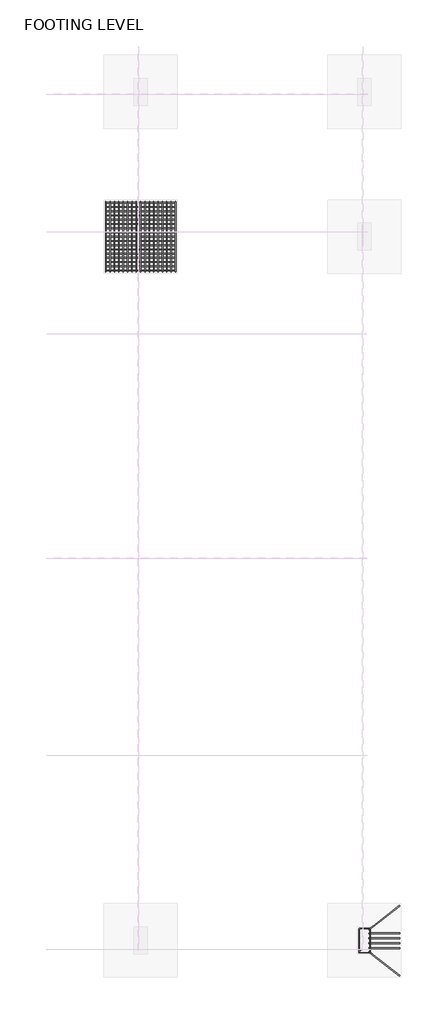
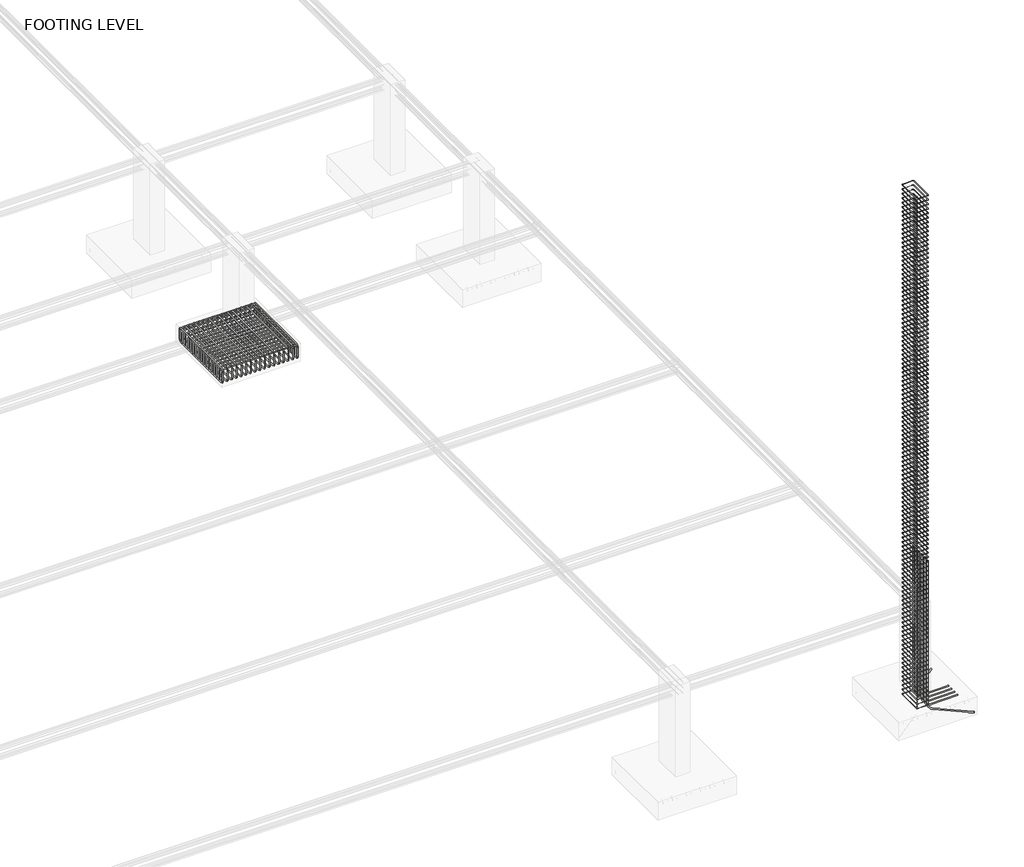
# One storey, part 9 of 19: 7 reinforcing bars.
"""IFC4 building model written with IfcOpenShell, lengths in millimetres."""

from ifc_helpers import new_model, si_unit, point, frame, origin, place, context, project, spatial, polyline, circle_curve, trimmed, segment, composite_curve, source, transform, mapped, element, save
from ifc_brep_helpers import swept_disk

model = new_model("IFC4")

# Units and contexts
model_context = context("Model", 3, world=origin())
ifc_project = project(units=[si_unit("LENGTHUNIT", "METRE", prefix="MILLI")], contexts=[model_context])

# Site, building, storey
site = spatial("IfcSite", under=ifc_project)
building = spatial("IfcBuilding", under=site)
storey = spatial("IfcBuildingStorey", under=building, Name="FOOTING LEVEL", Elevation=-3048.0)

# Reinforcing bars
placement = place(None, origin())
element("IfcReinforcingBar", 1, at=placement, inside=storey, context=model_context, shape_type="SolidModel", body=[
    swept_disk(composite_curve([segment(polyline([(32474.4469298, -27441.1521798, 1397.9656204), (32474.4469298, -27441.1521798, -3426.35)]), True, "CONTINUOUS"), segment(trimmed(circle_curve(frame((32595.5247821, -27346.5557941, -3426.35), z_axis=(0.6156614753256462, -0.7880107536067313, 0.0), x_axis=(-121.07785230000081, -94.59638569999879, 0.0)), 153.65), [point((32474.4469298, -27441.1521798, -3426.35))], [point((32595.5247821, -27346.5557941, -3580.0))], True, "CARTESIAN"), True, "CONTINUOUS"), segment(polyline([(32595.5247821, -27346.5557941, -3580.0), (33499.706152, -26640.131886, -3580.0)]), True, "CONTINUOUS")], self_intersect=False), 16.15),
])
element("IfcReinforcingBar", 2, at=placement, inside=storey, context=model_context, shape_type="SolidModel", body=[
    swept_disk(composite_curve([segment(polyline([(32473.5341356, -28221.1523853, 1369.4444311), (32473.5341356, -28221.1523853, -3426.35)]), True, "CONTINUOUS"), segment(trimmed(circle_curve(frame((32594.6119879, -28315.7487709, -3426.35), z_axis=(-0.6156614753256462, -0.7880107536067313, 0.0), x_axis=(-121.07785230000081, 94.59638560000167, 0.0)), 153.65), [point((32473.5341356, -28221.1523853, -3426.35))], [point((32594.6119879, -28315.7487709, -3580.0))], True, "CARTESIAN"), True, "CONTINUOUS"), segment(polyline([(32594.6119879, -28315.7487709, -3580.0), (33498.456152, -29021.9092249, -3580.0)]), True, "CONTINUOUS")], self_intersect=False), 16.15),
])
reinforcing_bar_shape = source(origin(), model_context, "Body", "SolidModel", [
    swept_disk(composite_curve([segment(polyline([(32475.5087563, -28081.7876394, 1399.9726557), (32475.5087563, -28081.7876394, -3426.35)]), True, "CONTINUOUS"), segment(trimmed(circle_curve(frame((32629.1587563, -28081.7876394, -3426.35), z_axis=(0.0, -1.0, 0.0), x_axis=(-153.64999999999782, 0.0, 0.0)), 153.65), [point((32475.5087563, -28081.7876394, -3426.35))], [point((32629.1587563, -28081.7876394, -3580.0))], True, "CARTESIAN"), True, "CONTINUOUS"), segment(polyline([(32629.1587563, -28081.7876394, -3580.0), (33512.5587563, -28081.7876394, -3580.0)]), True, "CONTINUOUS")], self_intersect=False), 16.15),
])
element("IfcReinforcingBar", 3, at=placement, inside=storey, context=model_context, shape_type="MappedRepresentation", body=[
    mapped(reinforcing_bar_shape, transform((0.0, 0.0, 0.0), x_axis=(1.0, 0.0, 0.0), y_axis=(0.0, 1.0, 0.0), z_axis=(0.0, 0.0, 1.0))),
    mapped(reinforcing_bar_shape, transform((0.0, 165.6818922, 0.0), x_axis=(1.0, 0.0, 0.0), y_axis=(0.0, 1.0, 0.0), z_axis=(0.0, 0.0, 1.0))),
    mapped(reinforcing_bar_shape, transform((0.0, 331.3637844, 0.0), x_axis=(1.0, 0.0, 0.0), y_axis=(0.0, 1.0, 0.0), z_axis=(0.0, 0.0, 1.0))),
    mapped(reinforcing_bar_shape, transform((0.0, 497.0456766, 0.0), x_axis=(1.0, 0.0, 0.0), y_axis=(0.0, 1.0, 0.0), z_axis=(0.0, 0.0, 1.0))),
])
reinforcing_bar_2_shape = source(origin(), model_context, "Body", "SolidModel", [
    swept_disk(composite_curve([segment(polyline([(32193.3637521, -28143.8137739, -3453.7796924), (32135.9578634, -28201.2196626, -3453.7796924)]), True, "CONTINUOUS"), segment(trimmed(circle_curve(frame((32153.4587563, -28218.7205555, -3453.7796924), z_axis=(0.0, 0.0, 1.0), x_axis=(-17.5008928999996, 17.5008928999996, 0.0)), 24.75), [point((32135.9578634, -28201.2196626, -3453.7796924))], [point((32153.4587563, -28243.4705555, -3453.7796924))], True, "CARTESIAN"), True, "CONTINUOUS"), segment(polyline([(32153.4587563, -28243.4705555, -3453.7796924), (32471.6587563, -28243.4705555, -3453.7796924)]), True, "CONTINUOUS"), segment(trimmed(circle_curve(frame((32471.6587563, -28218.7205555, -3453.7796924), z_axis=(0.0, 0.0, 1.0), x_axis=(0.0, -24.75, 0.0)), 24.75), [point((32471.6587563, -28243.4705555, -3453.7796924))], [point((32496.4087563, -28218.7205555, -3453.7796924))], True, "CARTESIAN"), True, "CONTINUOUS"), segment(polyline([(32496.4087563, -28218.7205555, -3453.7796924), (32496.4087563, -27443.3205555, -3453.7796924)]), True, "CONTINUOUS"), segment(trimmed(circle_curve(frame((32471.6670126, -27443.3205555, -3454.418927), z_axis=(-0.025827660859665615, 0.0, 0.9996664103262238), x_axis=(24.74174370000037, 0.0, 0.6392346000002362)), 24.75), [point((32496.4087563, -27443.3205555, -3453.7796924))], [point((32471.6670126, -27418.5705555, -3454.418927))], True, "CARTESIAN"), True, "CONTINUOUS"), segment(polyline([(32471.6670126, -27418.5705555, -3454.418927), (32153.4504999, -27418.5705555, -3462.6404578)]), True, "CONTINUOUS"), segment(trimmed(circle_curve(frame((32153.4504999, -27443.3205555, -3462.6404578), z_axis=(-0.025827660859665615, 0.0, 0.9996664103262238), x_axis=(0.0, 24.75, 0.0)), 24.75), [point((32153.4504999, -27418.5705555, -3462.6404578))], [point((32128.7087563, -27443.3205555, -3463.2796924))], True, "CARTESIAN"), True, "CONTINUOUS"), segment(polyline([(32128.7087563, -27443.3205555, -3463.2796924), (32128.7087563, -28248.2205555, -3463.2796924)]), True, "CONTINUOUS")], self_intersect=False), 4.75),
])
element("IfcReinforcingBar", 4, at=placement, inside=storey, context=model_context, shape_type="MappedRepresentation", body=[
    mapped(reinforcing_bar_2_shape, transform((0.0, 0.0, 0.0), x_axis=(1.0, 0.0, 0.0), y_axis=(0.0, 1.0, 0.0), z_axis=(0.0, 0.0, 1.0))),
    mapped(reinforcing_bar_2_shape, transform((0.0, 0.0, 149.7677811), x_axis=(1.0, 0.0, 0.0), y_axis=(0.0, 1.0, 0.0), z_axis=(0.0, 0.0, 1.0))),
    mapped(reinforcing_bar_2_shape, transform((0.0, 0.0, 299.5355623), x_axis=(1.0, 0.0, 0.0), y_axis=(0.0, 1.0, 0.0), z_axis=(0.0, 0.0, 1.0))),
    mapped(reinforcing_bar_2_shape, transform((0.0, 0.0, 449.3033434), x_axis=(1.0, 0.0, 0.0), y_axis=(0.0, 1.0, 0.0), z_axis=(0.0, 0.0, 1.0))),
    mapped(reinforcing_bar_2_shape, transform((0.0, 0.0, 599.0711246), x_axis=(1.0, 0.0, 0.0), y_axis=(0.0, 1.0, 0.0), z_axis=(0.0, 0.0, 1.0))),
    mapped(reinforcing_bar_2_shape, transform((0.0, 0.0, 748.8389057), x_axis=(1.0, 0.0, 0.0), y_axis=(0.0, 1.0, 0.0), z_axis=(0.0, 0.0, 1.0))),
    mapped(reinforcing_bar_2_shape, transform((0.0, 0.0, 898.6066869), x_axis=(1.0, 0.0, 0.0), y_axis=(0.0, 1.0, 0.0), z_axis=(0.0, 0.0, 1.0))),
    mapped(reinforcing_bar_2_shape, transform((0.0, 0.0, 1048.374468), x_axis=(1.0, 0.0, 0.0), y_axis=(0.0, 1.0, 0.0), z_axis=(0.0, 0.0, 1.0))),
    mapped(reinforcing_bar_2_shape, transform((0.0, 0.0, 1198.1422492), x_axis=(1.0, 0.0, 0.0), y_axis=(0.0, 1.0, 0.0), z_axis=(0.0, 0.0, 1.0))),
    mapped(reinforcing_bar_2_shape, transform((0.0, 0.0, 1347.9100303), x_axis=(1.0, 0.0, 0.0), y_axis=(0.0, 1.0, 0.0), z_axis=(0.0, 0.0, 1.0))),
    mapped(reinforcing_bar_2_shape, transform((0.0, 0.0, 1497.6778114), x_axis=(1.0, 0.0, 0.0), y_axis=(0.0, 1.0, 0.0), z_axis=(0.0, 0.0, 1.0))),
    mapped(reinforcing_bar_2_shape, transform((0.0, 0.0, 1647.4455926), x_axis=(1.0, 0.0, 0.0), y_axis=(0.0, 1.0, 0.0), z_axis=(0.0, 0.0, 1.0))),
    mapped(reinforcing_bar_2_shape, transform((0.0, 0.0, 1797.2133737), x_axis=(1.0, 0.0, 0.0), y_axis=(0.0, 1.0, 0.0), z_axis=(0.0, 0.0, 1.0))),
    mapped(reinforcing_bar_2_shape, transform((0.0, 0.0, 1946.9811549), x_axis=(1.0, 0.0, 0.0), y_axis=(0.0, 1.0, 0.0), z_axis=(0.0, 0.0, 1.0))),
    mapped(reinforcing_bar_2_shape, transform((0.0, 0.0, 2096.748936), x_axis=(1.0, 0.0, 0.0), y_axis=(0.0, 1.0, 0.0), z_axis=(0.0, 0.0, 1.0))),
    mapped(reinforcing_bar_2_shape, transform((0.0, 0.0, 2246.5167172), x_axis=(1.0, 0.0, 0.0), y_axis=(0.0, 1.0, 0.0), z_axis=(0.0, 0.0, 1.0))),
    mapped(reinforcing_bar_2_shape, transform((0.0, 0.0, 2396.2844983), x_axis=(1.0, 0.0, 0.0), y_axis=(0.0, 1.0, 0.0), z_axis=(0.0, 0.0, 1.0))),
    mapped(reinforcing_bar_2_shape, transform((0.0, 0.0, 2546.0522795), x_axis=(1.0, 0.0, 0.0), y_axis=(0.0, 1.0, 0.0), z_axis=(0.0, 0.0, 1.0))),
    mapped(reinforcing_bar_2_shape, transform((0.0, 0.0, 2695.8200606), x_axis=(1.0, 0.0, 0.0), y_axis=(0.0, 1.0, 0.0), z_axis=(0.0, 0.0, 1.0))),
    mapped(reinforcing_bar_2_shape, transform((0.0, 0.0, 2845.5878418), x_axis=(1.0, 0.0, 0.0), y_axis=(0.0, 1.0, 0.0), z_axis=(0.0, 0.0, 1.0))),
    mapped(reinforcing_bar_2_shape, transform((0.0, 0.0, 2995.3556229), x_axis=(1.0, 0.0, 0.0), y_axis=(0.0, 1.0, 0.0), z_axis=(0.0, 0.0, 1.0))),
    mapped(reinforcing_bar_2_shape, transform((0.0, 0.0, 3145.123404), x_axis=(1.0, 0.0, 0.0), y_axis=(0.0, 1.0, 0.0), z_axis=(0.0, 0.0, 1.0))),
    mapped(reinforcing_bar_2_shape, transform((0.0, 0.0, 3294.8911852), x_axis=(1.0, 0.0, 0.0), y_axis=(0.0, 1.0, 0.0), z_axis=(0.0, 0.0, 1.0))),
    mapped(reinforcing_bar_2_shape, transform((0.0, 0.0, 3444.6589663), x_axis=(1.0, 0.0, 0.0), y_axis=(0.0, 1.0, 0.0), z_axis=(0.0, 0.0, 1.0))),
    mapped(reinforcing_bar_2_shape, transform((0.0, 0.0, 3594.4267475), x_axis=(1.0, 0.0, 0.0), y_axis=(0.0, 1.0, 0.0), z_axis=(0.0, 0.0, 1.0))),
    mapped(reinforcing_bar_2_shape, transform((0.0, 0.0, 3744.1945286), x_axis=(1.0, 0.0, 0.0), y_axis=(0.0, 1.0, 0.0), z_axis=(0.0, 0.0, 1.0))),
    mapped(reinforcing_bar_2_shape, transform((0.0, 0.0, 3893.9623098), x_axis=(1.0, 0.0, 0.0), y_axis=(0.0, 1.0, 0.0), z_axis=(0.0, 0.0, 1.0))),
    mapped(reinforcing_bar_2_shape, transform((0.0, 0.0, 4043.7300909), x_axis=(1.0, 0.0, 0.0), y_axis=(0.0, 1.0, 0.0), z_axis=(0.0, 0.0, 1.0))),
    mapped(reinforcing_bar_2_shape, transform((0.0, 0.0, 4193.4978721), x_axis=(1.0, 0.0, 0.0), y_axis=(0.0, 1.0, 0.0), z_axis=(0.0, 0.0, 1.0))),
    mapped(reinforcing_bar_2_shape, transform((0.0, 0.0, 4343.2656532), x_axis=(1.0, 0.0, 0.0), y_axis=(0.0, 1.0, 0.0), z_axis=(0.0, 0.0, 1.0))),
    mapped(reinforcing_bar_2_shape, transform((0.0, 0.0, 4493.0334343), x_axis=(1.0, 0.0, 0.0), y_axis=(0.0, 1.0, 0.0), z_axis=(0.0, 0.0, 1.0))),
    mapped(reinforcing_bar_2_shape, transform((0.0, 0.0, 4642.8012155), x_axis=(1.0, 0.0, 0.0), y_axis=(0.0, 1.0, 0.0), z_axis=(0.0, 0.0, 1.0))),
    mapped(reinforcing_bar_2_shape, transform((0.0, 0.0, 4792.5689966), x_axis=(1.0, 0.0, 0.0), y_axis=(0.0, 1.0, 0.0), z_axis=(0.0, 0.0, 1.0))),
    mapped(reinforcing_bar_2_shape, transform((0.0, 0.0, 4942.3367778), x_axis=(1.0, 0.0, 0.0), y_axis=(0.0, 1.0, 0.0), z_axis=(0.0, 0.0, 1.0))),
    mapped(reinforcing_bar_2_shape, transform((0.0, 0.0, 5092.1045589), x_axis=(1.0, 0.0, 0.0), y_axis=(0.0, 1.0, 0.0), z_axis=(0.0, 0.0, 1.0))),
    mapped(reinforcing_bar_2_shape, transform((0.0, 0.0, 5241.8723401), x_axis=(1.0, 0.0, 0.0), y_axis=(0.0, 1.0, 0.0), z_axis=(0.0, 0.0, 1.0))),
    mapped(reinforcing_bar_2_shape, transform((0.0, 0.0, 5391.6401212), x_axis=(1.0, 0.0, 0.0), y_axis=(0.0, 1.0, 0.0), z_axis=(0.0, 0.0, 1.0))),
    mapped(reinforcing_bar_2_shape, transform((0.0, 0.0, 5541.4079024), x_axis=(1.0, 0.0, 0.0), y_axis=(0.0, 1.0, 0.0), z_axis=(0.0, 0.0, 1.0))),
    mapped(reinforcing_bar_2_shape, transform((0.0, 0.0, 5691.1756835), x_axis=(1.0, 0.0, 0.0), y_axis=(0.0, 1.0, 0.0), z_axis=(0.0, 0.0, 1.0))),
    mapped(reinforcing_bar_2_shape, transform((0.0, 0.0, 5840.9434646), x_axis=(1.0, 0.0, 0.0), y_axis=(0.0, 1.0, 0.0), z_axis=(0.0, 0.0, 1.0))),
    mapped(reinforcing_bar_2_shape, transform((0.0, 0.0, 5990.7112458), x_axis=(1.0, 0.0, 0.0), y_axis=(0.0, 1.0, 0.0), z_axis=(0.0, 0.0, 1.0))),
    mapped(reinforcing_bar_2_shape, transform((0.0, 0.0, 6140.4790269), x_axis=(1.0, 0.0, 0.0), y_axis=(0.0, 1.0, 0.0), z_axis=(0.0, 0.0, 1.0))),
    mapped(reinforcing_bar_2_shape, transform((0.0, 0.0, 6290.2468081), x_axis=(1.0, 0.0, 0.0), y_axis=(0.0, 1.0, 0.0), z_axis=(0.0, 0.0, 1.0))),
    mapped(reinforcing_bar_2_shape, transform((0.0, 0.0, 6440.0145892), x_axis=(1.0, 0.0, 0.0), y_axis=(0.0, 1.0, 0.0), z_axis=(0.0, 0.0, 1.0))),
    mapped(reinforcing_bar_2_shape, transform((0.0, 0.0, 6589.7823704), x_axis=(1.0, 0.0, 0.0), y_axis=(0.0, 1.0, 0.0), z_axis=(0.0, 0.0, 1.0))),
    mapped(reinforcing_bar_2_shape, transform((0.0, 0.0, 6739.5501515), x_axis=(1.0, 0.0, 0.0), y_axis=(0.0, 1.0, 0.0), z_axis=(0.0, 0.0, 1.0))),
    mapped(reinforcing_bar_2_shape, transform((0.0, 0.0, 6889.3179327), x_axis=(1.0, 0.0, 0.0), y_axis=(0.0, 1.0, 0.0), z_axis=(0.0, 0.0, 1.0))),
    mapped(reinforcing_bar_2_shape, transform((0.0, 0.0, 7039.0857138), x_axis=(1.0, 0.0, 0.0), y_axis=(0.0, 1.0, 0.0), z_axis=(0.0, 0.0, 1.0))),
    mapped(reinforcing_bar_2_shape, transform((0.0, 0.0, 7188.853495), x_axis=(1.0, 0.0, 0.0), y_axis=(0.0, 1.0, 0.0), z_axis=(0.0, 0.0, 1.0))),
    mapped(reinforcing_bar_2_shape, transform((0.0, 0.0, 7338.6212761), x_axis=(1.0, 0.0, 0.0), y_axis=(0.0, 1.0, 0.0), z_axis=(0.0, 0.0, 1.0))),
    mapped(reinforcing_bar_2_shape, transform((0.0, 0.0, 7488.3890572), x_axis=(1.0, 0.0, 0.0), y_axis=(0.0, 1.0, 0.0), z_axis=(0.0, 0.0, 1.0))),
    mapped(reinforcing_bar_2_shape, transform((0.0, 0.0, 7638.1568384), x_axis=(1.0, 0.0, 0.0), y_axis=(0.0, 1.0, 0.0), z_axis=(0.0, 0.0, 1.0))),
    mapped(reinforcing_bar_2_shape, transform((0.0, 0.0, 7787.9246195), x_axis=(1.0, 0.0, 0.0), y_axis=(0.0, 1.0, 0.0), z_axis=(0.0, 0.0, 1.0))),
    mapped(reinforcing_bar_2_shape, transform((0.0, 0.0, 7937.6924007), x_axis=(1.0, 0.0, 0.0), y_axis=(0.0, 1.0, 0.0), z_axis=(0.0, 0.0, 1.0))),
    mapped(reinforcing_bar_2_shape, transform((0.0, 0.0, 8087.4601818), x_axis=(1.0, 0.0, 0.0), y_axis=(0.0, 1.0, 0.0), z_axis=(0.0, 0.0, 1.0))),
    mapped(reinforcing_bar_2_shape, transform((0.0, 0.0, 8237.227963), x_axis=(1.0, 0.0, 0.0), y_axis=(0.0, 1.0, 0.0), z_axis=(0.0, 0.0, 1.0))),
    mapped(reinforcing_bar_2_shape, transform((0.0, 0.0, 8386.9957441), x_axis=(1.0, 0.0, 0.0), y_axis=(0.0, 1.0, 0.0), z_axis=(0.0, 0.0, 1.0))),
    mapped(reinforcing_bar_2_shape, transform((0.0, 0.0, 8536.7635253), x_axis=(1.0, 0.0, 0.0), y_axis=(0.0, 1.0, 0.0), z_axis=(0.0, 0.0, 1.0))),
    mapped(reinforcing_bar_2_shape, transform((0.0, 0.0, 8686.5313064), x_axis=(1.0, 0.0, 0.0), y_axis=(0.0, 1.0, 0.0), z_axis=(0.0, 0.0, 1.0))),
    mapped(reinforcing_bar_2_shape, transform((0.0, 0.0, 8836.2990875), x_axis=(1.0, 0.0, 0.0), y_axis=(0.0, 1.0, 0.0), z_axis=(0.0, 0.0, 1.0))),
    mapped(reinforcing_bar_2_shape, transform((0.0, 0.0, 8986.0668687), x_axis=(1.0, 0.0, 0.0), y_axis=(0.0, 1.0, 0.0), z_axis=(0.0, 0.0, 1.0))),
    mapped(reinforcing_bar_2_shape, transform((0.0, 0.0, 9135.8346498), x_axis=(1.0, 0.0, 0.0), y_axis=(0.0, 1.0, 0.0), z_axis=(0.0, 0.0, 1.0))),
    mapped(reinforcing_bar_2_shape, transform((0.0, 0.0, 9285.602431), x_axis=(1.0, 0.0, 0.0), y_axis=(0.0, 1.0, 0.0), z_axis=(0.0, 0.0, 1.0))),
    mapped(reinforcing_bar_2_shape, transform((0.0, 0.0, 9435.3702121), x_axis=(1.0, 0.0, 0.0), y_axis=(0.0, 1.0, 0.0), z_axis=(0.0, 0.0, 1.0))),
    mapped(reinforcing_bar_2_shape, transform((0.0, 0.0, 9585.1379933), x_axis=(1.0, 0.0, 0.0), y_axis=(0.0, 1.0, 0.0), z_axis=(0.0, 0.0, 1.0))),
    mapped(reinforcing_bar_2_shape, transform((0.0, 0.0, 9734.9057744), x_axis=(1.0, 0.0, 0.0), y_axis=(0.0, 1.0, 0.0), z_axis=(0.0, 0.0, 1.0))),
    mapped(reinforcing_bar_2_shape, transform((0.0, 0.0, 9884.6735556), x_axis=(1.0, 0.0, 0.0), y_axis=(0.0, 1.0, 0.0), z_axis=(0.0, 0.0, 1.0))),
    mapped(reinforcing_bar_2_shape, transform((0.0, 0.0, 10034.4413367), x_axis=(1.0, 0.0, 0.0), y_axis=(0.0, 1.0, 0.0), z_axis=(0.0, 0.0, 1.0))),
    mapped(reinforcing_bar_2_shape, transform((0.0, 0.0, 10184.2091178), x_axis=(1.0, 0.0, 0.0), y_axis=(0.0, 1.0, 0.0), z_axis=(0.0, 0.0, 1.0))),
    mapped(reinforcing_bar_2_shape, transform((0.0, 0.0, 10333.976899), x_axis=(1.0, 0.0, 0.0), y_axis=(0.0, 1.0, 0.0), z_axis=(0.0, 0.0, 1.0))),
    mapped(reinforcing_bar_2_shape, transform((0.0, 0.0, 10483.7446801), x_axis=(1.0, 0.0, 0.0), y_axis=(0.0, 1.0, 0.0), z_axis=(0.0, 0.0, 1.0))),
    mapped(reinforcing_bar_2_shape, transform((0.0, 0.0, 10633.5124613), x_axis=(1.0, 0.0, 0.0), y_axis=(0.0, 1.0, 0.0), z_axis=(0.0, 0.0, 1.0))),
    mapped(reinforcing_bar_2_shape, transform((0.0, 0.0, 10783.2802424), x_axis=(1.0, 0.0, 0.0), y_axis=(0.0, 1.0, 0.0), z_axis=(0.0, 0.0, 1.0))),
    mapped(reinforcing_bar_2_shape, transform((0.0, 0.0, 10933.0480236), x_axis=(1.0, 0.0, 0.0), y_axis=(0.0, 1.0, 0.0), z_axis=(0.0, 0.0, 1.0))),
    mapped(reinforcing_bar_2_shape, transform((0.0, 0.0, 11082.8158047), x_axis=(1.0, 0.0, 0.0), y_axis=(0.0, 1.0, 0.0), z_axis=(0.0, 0.0, 1.0))),
    mapped(reinforcing_bar_2_shape, transform((0.0, 0.0, 11232.5835859), x_axis=(1.0, 0.0, 0.0), y_axis=(0.0, 1.0, 0.0), z_axis=(0.0, 0.0, 1.0))),
    mapped(reinforcing_bar_2_shape, transform((0.0, 0.0, 11382.351367), x_axis=(1.0, 0.0, 0.0), y_axis=(0.0, 1.0, 0.0), z_axis=(0.0, 0.0, 1.0))),
    mapped(reinforcing_bar_2_shape, transform((0.0, 0.0, 11532.1191482), x_axis=(1.0, 0.0, 0.0), y_axis=(0.0, 1.0, 0.0), z_axis=(0.0, 0.0, 1.0))),
    mapped(reinforcing_bar_2_shape, transform((0.0, 0.0, 11681.8869293), x_axis=(1.0, 0.0, 0.0), y_axis=(0.0, 1.0, 0.0), z_axis=(0.0, 0.0, 1.0))),
    mapped(reinforcing_bar_2_shape, transform((0.0, 0.0, 11831.6547104), x_axis=(1.0, 0.0, 0.0), y_axis=(0.0, 1.0, 0.0), z_axis=(0.0, 0.0, 1.0))),
    mapped(reinforcing_bar_2_shape, transform((0.0, 0.0, 11981.4224916), x_axis=(1.0, 0.0, 0.0), y_axis=(0.0, 1.0, 0.0), z_axis=(0.0, 0.0, 1.0))),
    mapped(reinforcing_bar_2_shape, transform((0.0, 0.0, 12131.1902727), x_axis=(1.0, 0.0, 0.0), y_axis=(0.0, 1.0, 0.0), z_axis=(0.0, 0.0, 1.0))),
    mapped(reinforcing_bar_2_shape, transform((0.0, 0.0, 12280.9580539), x_axis=(1.0, 0.0, 0.0), y_axis=(0.0, 1.0, 0.0), z_axis=(0.0, 0.0, 1.0))),
    mapped(reinforcing_bar_2_shape, transform((0.0, 0.0, 12430.725835), x_axis=(1.0, 0.0, 0.0), y_axis=(0.0, 1.0, 0.0), z_axis=(0.0, 0.0, 1.0))),
    mapped(reinforcing_bar_2_shape, transform((0.0, 0.0, 12580.4936162), x_axis=(1.0, 0.0, 0.0), y_axis=(0.0, 1.0, 0.0), z_axis=(0.0, 0.0, 1.0))),
    mapped(reinforcing_bar_2_shape, transform((0.0, 0.0, 12730.2613973), x_axis=(1.0, 0.0, 0.0), y_axis=(0.0, 1.0, 0.0), z_axis=(0.0, 0.0, 1.0))),
    mapped(reinforcing_bar_2_shape, transform((0.0, 0.0, 12880.0291785), x_axis=(1.0, 0.0, 0.0), y_axis=(0.0, 1.0, 0.0), z_axis=(0.0, 0.0, 1.0))),
    mapped(reinforcing_bar_2_shape, transform((0.0, 0.0, 13029.7969596), x_axis=(1.0, 0.0, 0.0), y_axis=(0.0, 1.0, 0.0), z_axis=(0.0, 0.0, 1.0))),
    mapped(reinforcing_bar_2_shape, transform((0.0, 0.0, 13179.5647407), x_axis=(1.0, 0.0, 0.0), y_axis=(0.0, 1.0, 0.0), z_axis=(0.0, 0.0, 1.0))),
    mapped(reinforcing_bar_2_shape, transform((0.0, 0.0, 13329.3325219), x_axis=(1.0, 0.0, 0.0), y_axis=(0.0, 1.0, 0.0), z_axis=(0.0, 0.0, 1.0))),
    mapped(reinforcing_bar_2_shape, transform((0.0, 0.0, 13479.100303), x_axis=(1.0, 0.0, 0.0), y_axis=(0.0, 1.0, 0.0), z_axis=(0.0, 0.0, 1.0))),
    mapped(reinforcing_bar_2_shape, transform((0.0, 0.0, 13628.8680842), x_axis=(1.0, 0.0, 0.0), y_axis=(0.0, 1.0, 0.0), z_axis=(0.0, 0.0, 1.0))),
    mapped(reinforcing_bar_2_shape, transform((0.0, 0.0, 13778.6358653), x_axis=(1.0, 0.0, 0.0), y_axis=(0.0, 1.0, 0.0), z_axis=(0.0, 0.0, 1.0))),
    mapped(reinforcing_bar_2_shape, transform((0.0, 0.0, 13928.4036465), x_axis=(1.0, 0.0, 0.0), y_axis=(0.0, 1.0, 0.0), z_axis=(0.0, 0.0, 1.0))),
    mapped(reinforcing_bar_2_shape, transform((0.0, 0.0, 14078.1714276), x_axis=(1.0, 0.0, 0.0), y_axis=(0.0, 1.0, 0.0), z_axis=(0.0, 0.0, 1.0))),
    mapped(reinforcing_bar_2_shape, transform((0.0, 0.0, 14227.9392088), x_axis=(1.0, 0.0, 0.0), y_axis=(0.0, 1.0, 0.0), z_axis=(0.0, 0.0, 1.0))),
    mapped(reinforcing_bar_2_shape, transform((0.0, 0.0, 14377.7069899), x_axis=(1.0, 0.0, 0.0), y_axis=(0.0, 1.0, 0.0), z_axis=(0.0, 0.0, 1.0))),
    mapped(reinforcing_bar_2_shape, transform((0.0, 0.0, 14527.474771), x_axis=(1.0, 0.0, 0.0), y_axis=(0.0, 1.0, 0.0), z_axis=(0.0, 0.0, 1.0))),
    mapped(reinforcing_bar_2_shape, transform((0.0, 0.0, 14677.2425522), x_axis=(1.0, 0.0, 0.0), y_axis=(0.0, 1.0, 0.0), z_axis=(0.0, 0.0, 1.0))),
    mapped(reinforcing_bar_2_shape, transform((0.0, 0.0, 14827.0103333), x_axis=(1.0, 0.0, 0.0), y_axis=(0.0, 1.0, 0.0), z_axis=(0.0, 0.0, 1.0))),
    mapped(reinforcing_bar_2_shape, transform((0.0, 0.0, 14976.7781145), x_axis=(1.0, 0.0, 0.0), y_axis=(0.0, 1.0, 0.0), z_axis=(0.0, 0.0, 1.0))),
    mapped(reinforcing_bar_2_shape, transform((0.0, 0.0, 15126.5458956), x_axis=(1.0, 0.0, 0.0), y_axis=(0.0, 1.0, 0.0), z_axis=(0.0, 0.0, 1.0))),
    mapped(reinforcing_bar_2_shape, transform((0.0, 0.0, 15276.3136768), x_axis=(1.0, 0.0, 0.0), y_axis=(0.0, 1.0, 0.0), z_axis=(0.0, 0.0, 1.0))),
    mapped(reinforcing_bar_2_shape, transform((0.0, 0.0, 15426.0814579), x_axis=(1.0, 0.0, 0.0), y_axis=(0.0, 1.0, 0.0), z_axis=(0.0, 0.0, 1.0))),
    mapped(reinforcing_bar_2_shape, transform((0.0, 0.0, 15575.8492391), x_axis=(1.0, 0.0, 0.0), y_axis=(0.0, 1.0, 0.0), z_axis=(0.0, 0.0, 1.0))),
    mapped(reinforcing_bar_2_shape, transform((0.0, 0.0, 15725.6170202), x_axis=(1.0, 0.0, 0.0), y_axis=(0.0, 1.0, 0.0), z_axis=(0.0, 0.0, 1.0))),
    mapped(reinforcing_bar_2_shape, transform((0.0, 0.0, 15875.3848014), x_axis=(1.0, 0.0, 0.0), y_axis=(0.0, 1.0, 0.0), z_axis=(0.0, 0.0, 1.0))),
    mapped(reinforcing_bar_2_shape, transform((0.0, 0.0, 16025.1525825), x_axis=(1.0, 0.0, 0.0), y_axis=(0.0, 1.0, 0.0), z_axis=(0.0, 0.0, 1.0))),
    mapped(reinforcing_bar_2_shape, transform((0.0, 0.0, 16174.9203636), x_axis=(1.0, 0.0, 0.0), y_axis=(0.0, 1.0, 0.0), z_axis=(0.0, 0.0, 1.0))),
    mapped(reinforcing_bar_2_shape, transform((0.0, 0.0, 16324.6881448), x_axis=(1.0, 0.0, 0.0), y_axis=(0.0, 1.0, 0.0), z_axis=(0.0, 0.0, 1.0))),
    mapped(reinforcing_bar_2_shape, transform((0.0, 0.0, 16474.4559259), x_axis=(1.0, 0.0, 0.0), y_axis=(0.0, 1.0, 0.0), z_axis=(0.0, 0.0, 1.0))),
    mapped(reinforcing_bar_2_shape, transform((0.0, 0.0, 16624.2237071), x_axis=(1.0, 0.0, 0.0), y_axis=(0.0, 1.0, 0.0), z_axis=(0.0, 0.0, 1.0))),
    mapped(reinforcing_bar_2_shape, transform((0.0, 0.0, 16773.9914882), x_axis=(1.0, 0.0, 0.0), y_axis=(0.0, 1.0, 0.0), z_axis=(0.0, 0.0, 1.0))),
    mapped(reinforcing_bar_2_shape, transform((0.0, 0.0, 16923.7592694), x_axis=(1.0, 0.0, 0.0), y_axis=(0.0, 1.0, 0.0), z_axis=(0.0, 0.0, 1.0))),
    mapped(reinforcing_bar_2_shape, transform((0.0, 0.0, 17073.5270505), x_axis=(1.0, 0.0, 0.0), y_axis=(0.0, 1.0, 0.0), z_axis=(0.0, 0.0, 1.0))),
])
reinforcing_bar_3_shape = source(origin(), model_context, "Body", "SolidModel", [
    swept_disk(composite_curve([segment(polyline([(25879.8587563, -2750.5596072, -3548.0), (25879.8587563, -2750.5596072, -3225.9)]), True, "CONTINUOUS"), segment(trimmed(circle_curve(frame((25789.6587563, -2750.5596072, -3225.9), z_axis=(0.0, -1.0, 0.0), x_axis=(90.20000000000073, 0.0, 0.0)), 90.2), [point((25879.8587563, -2750.5596072, -3225.9))], [point((25789.6587563, -2750.5596072, -3135.7))], True, "CARTESIAN"), True, "CONTINUOUS"), segment(polyline([(25789.6587563, -2750.5596072, -3135.7), (23595.4587563, -2750.5596072, -3135.7)]), True, "CONTINUOUS"), segment(trimmed(circle_curve(frame((23595.4587563, -2750.5596072, -3225.9), z_axis=(0.0, -1.0, 0.0), x_axis=(0.0, 0.0, 90.20000000000027)), 90.2), [point((23595.4587563, -2750.5596072, -3135.7))], [point((23505.2587563, -2750.5596072, -3225.9))], True, "CARTESIAN"), True, "CONTINUOUS"), segment(polyline([(23505.2587563, -2750.5596072, -3225.9), (23505.2587563, -2750.5596072, -3548.0)]), True, "CONTINUOUS")], self_intersect=False), 12.7),
])
element("IfcReinforcingBar", 5, at=placement, inside=storey, context=model_context, shape_type="MappedRepresentation", body=[
    mapped(reinforcing_bar_3_shape, transform((0.0, 0.0, 0.0), x_axis=(1.0, 0.0, 0.0), y_axis=(0.0, 1.0, 0.0), z_axis=(0.0, 0.0, 1.0))),
    mapped(reinforcing_bar_3_shape, transform((0.0, -143.8496077, 0.0), x_axis=(1.0, 0.0, 0.0), y_axis=(0.0, 1.0, 0.0), z_axis=(0.0, 0.0, 1.0))),
    mapped(reinforcing_bar_3_shape, transform((0.0, -287.6992155, 0.0), x_axis=(1.0, 0.0, 0.0), y_axis=(0.0, 1.0, 0.0), z_axis=(0.0, 0.0, 1.0))),
    mapped(reinforcing_bar_3_shape, transform((0.0, -431.5488232, 0.0), x_axis=(1.0, 0.0, 0.0), y_axis=(0.0, 1.0, 0.0), z_axis=(0.0, 0.0, 1.0))),
    mapped(reinforcing_bar_3_shape, transform((0.0, -575.398431, 0.0), x_axis=(1.0, 0.0, 0.0), y_axis=(0.0, 1.0, 0.0), z_axis=(0.0, 0.0, 1.0))),
    mapped(reinforcing_bar_3_shape, transform((0.0, -719.2480387, 0.0), x_axis=(1.0, 0.0, 0.0), y_axis=(0.0, 1.0, 0.0), z_axis=(0.0, 0.0, 1.0))),
    mapped(reinforcing_bar_3_shape, transform((0.0, -863.0976465, 0.0), x_axis=(1.0, 0.0, 0.0), y_axis=(0.0, 1.0, 0.0), z_axis=(0.0, 0.0, 1.0))),
    mapped(reinforcing_bar_3_shape, transform((0.0, -1006.9472542, 0.0), x_axis=(1.0, 0.0, 0.0), y_axis=(0.0, 1.0, 0.0), z_axis=(0.0, 0.0, 1.0))),
    mapped(reinforcing_bar_3_shape, transform((0.0, -1150.796862, 0.0), x_axis=(1.0, 0.0, 0.0), y_axis=(0.0, 1.0, 0.0), z_axis=(0.0, 0.0, 1.0))),
    mapped(reinforcing_bar_3_shape, transform((0.0, -1294.6464697, 0.0), x_axis=(1.0, 0.0, 0.0), y_axis=(0.0, 1.0, 0.0), z_axis=(0.0, 0.0, 1.0))),
    mapped(reinforcing_bar_3_shape, transform((0.0, -1438.4960775, 0.0), x_axis=(1.0, 0.0, 0.0), y_axis=(0.0, 1.0, 0.0), z_axis=(0.0, 0.0, 1.0))),
    mapped(reinforcing_bar_3_shape, transform((0.0, -1582.3456852, 0.0), x_axis=(1.0, 0.0, 0.0), y_axis=(0.0, 1.0, 0.0), z_axis=(0.0, 0.0, 1.0))),
    mapped(reinforcing_bar_3_shape, transform((0.0, -1726.195293, 0.0), x_axis=(1.0, 0.0, 0.0), y_axis=(0.0, 1.0, 0.0), z_axis=(0.0, 0.0, 1.0))),
    mapped(reinforcing_bar_3_shape, transform((0.0, -1870.0449007, 0.0), x_axis=(1.0, 0.0, 0.0), y_axis=(0.0, 1.0, 0.0), z_axis=(0.0, 0.0, 1.0))),
    mapped(reinforcing_bar_3_shape, transform((0.0, -2013.8945085, 0.0), x_axis=(1.0, 0.0, 0.0), y_axis=(0.0, 1.0, 0.0), z_axis=(0.0, 0.0, 1.0))),
    mapped(reinforcing_bar_3_shape, transform((0.0, -2157.7441162, 0.0), x_axis=(1.0, 0.0, 0.0), y_axis=(0.0, 1.0, 0.0), z_axis=(0.0, 0.0, 1.0))),
    mapped(reinforcing_bar_3_shape, transform((0.0, -2301.5937239, 0.0), x_axis=(1.0, 0.0, 0.0), y_axis=(0.0, 1.0, 0.0), z_axis=(0.0, 0.0, 1.0))),
])
reinforcing_bar_4_shape = source(origin(), model_context, "Body", "SolidModel", [
    swept_disk(composite_curve([segment(polyline([(23505.2587563, -5091.5205555, -3173.0), (23505.2587563, -5091.5205555, -3495.1)]), True, "CONTINUOUS"), segment(trimmed(circle_curve(frame((23505.2587563, -5001.3205555, -3495.1), z_axis=(1.0, 0.0, 0.0), x_axis=(0.0, -90.19999999999982, 0.0)), 90.2), [point((23505.2587563, -5091.5205555, -3495.1))], [point((23505.2587563, -5001.3205555, -3585.3))], True, "CARTESIAN"), True, "CONTINUOUS"), segment(polyline([(23505.2587563, -5001.3205555, -3585.3), (23505.2587563, -2807.1205555, -3585.3)]), True, "CONTINUOUS"), segment(trimmed(circle_curve(frame((23505.2587563, -2807.1205555, -3495.1), z_axis=(1.0, 0.0, 0.0), x_axis=(0.0, 0.0, -90.20000000000027)), 90.2), [point((23505.2587563, -2807.1205555, -3585.3))], [point((23505.2587563, -2716.9205555, -3495.1))], True, "CARTESIAN"), True, "CONTINUOUS"), segment(polyline([(23505.2587563, -2716.9205555, -3495.1), (23505.2587563, -2716.9205555, -3173.0)]), True, "CONTINUOUS")], self_intersect=False), 12.7),
])
element("IfcReinforcingBar", 6, at=placement, inside=storey, context=model_context, shape_type="MappedRepresentation", body=[
    mapped(reinforcing_bar_4_shape, transform((0.0, 0.0, 0.0), x_axis=(1.0, 0.0, 0.0), y_axis=(0.0, 1.0, 0.0), z_axis=(0.0, 0.0, 1.0))),
    mapped(reinforcing_bar_4_shape, transform((148.4125, 0.0, 0.0), x_axis=(1.0, 0.0, 0.0), y_axis=(0.0, 1.0, 0.0), z_axis=(0.0, 0.0, 1.0))),
    mapped(reinforcing_bar_4_shape, transform((296.825, 0.0, 0.0), x_axis=(1.0, 0.0, 0.0), y_axis=(0.0, 1.0, 0.0), z_axis=(0.0, 0.0, 1.0))),
    mapped(reinforcing_bar_4_shape, transform((445.2375, 0.0, 0.0), x_axis=(1.0, 0.0, 0.0), y_axis=(0.0, 1.0, 0.0), z_axis=(0.0, 0.0, 1.0))),
    mapped(reinforcing_bar_4_shape, transform((593.65, 0.0, 0.0), x_axis=(1.0, 0.0, 0.0), y_axis=(0.0, 1.0, 0.0), z_axis=(0.0, 0.0, 1.0))),
    mapped(reinforcing_bar_4_shape, transform((742.0625, 0.0, 0.0), x_axis=(1.0, 0.0, 0.0), y_axis=(0.0, 1.0, 0.0), z_axis=(0.0, 0.0, 1.0))),
    mapped(reinforcing_bar_4_shape, transform((890.475, 0.0, 0.0), x_axis=(1.0, 0.0, 0.0), y_axis=(0.0, 1.0, 0.0), z_axis=(0.0, 0.0, 1.0))),
    mapped(reinforcing_bar_4_shape, transform((1038.8875, 0.0, 0.0), x_axis=(1.0, 0.0, 0.0), y_axis=(0.0, 1.0, 0.0), z_axis=(0.0, 0.0, 1.0))),
    mapped(reinforcing_bar_4_shape, transform((1187.3, 0.0, 0.0), x_axis=(1.0, 0.0, 0.0), y_axis=(0.0, 1.0, 0.0), z_axis=(0.0, 0.0, 1.0))),
    mapped(reinforcing_bar_4_shape, transform((1335.7125, 0.0, 0.0), x_axis=(1.0, 0.0, 0.0), y_axis=(0.0, 1.0, 0.0), z_axis=(0.0, 0.0, 1.0))),
    mapped(reinforcing_bar_4_shape, transform((1484.125, 0.0, 0.0), x_axis=(1.0, 0.0, 0.0), y_axis=(0.0, 1.0, 0.0), z_axis=(0.0, 0.0, 1.0))),
    mapped(reinforcing_bar_4_shape, transform((1632.5375, 0.0, 0.0), x_axis=(1.0, 0.0, 0.0), y_axis=(0.0, 1.0, 0.0), z_axis=(0.0, 0.0, 1.0))),
    mapped(reinforcing_bar_4_shape, transform((1780.95, 0.0, 0.0), x_axis=(1.0, 0.0, 0.0), y_axis=(0.0, 1.0, 0.0), z_axis=(0.0, 0.0, 1.0))),
    mapped(reinforcing_bar_4_shape, transform((1929.3625, 0.0, 0.0), x_axis=(1.0, 0.0, 0.0), y_axis=(0.0, 1.0, 0.0), z_axis=(0.0, 0.0, 1.0))),
    mapped(reinforcing_bar_4_shape, transform((2077.775, 0.0, 0.0), x_axis=(1.0, 0.0, 0.0), y_axis=(0.0, 1.0, 0.0), z_axis=(0.0, 0.0, 1.0))),
    mapped(reinforcing_bar_4_shape, transform((2226.1875, 0.0, 0.0), x_axis=(1.0, 0.0, 0.0), y_axis=(0.0, 1.0, 0.0), z_axis=(0.0, 0.0, 1.0))),
    mapped(reinforcing_bar_4_shape, transform((2374.6, 0.0, 0.0), x_axis=(1.0, 0.0, 0.0), y_axis=(0.0, 1.0, 0.0), z_axis=(0.0, 0.0, 1.0))),
])
reinforcing_bar_5_shape = source(origin(), model_context, "Body", "SolidModel", [
    swept_disk(composite_curve([segment(polyline([(23505.2587563, -2716.9205555, -3523.0), (23505.2587563, -2716.9205555, -3200.9)]), True, "CONTINUOUS"), segment(trimmed(circle_curve(frame((23505.2587563, -2807.1205555, -3200.9), z_axis=(1.0, 0.0, 0.0), x_axis=(0.0, 90.20000000000027, 0.0)), 90.2), [point((23505.2587563, -2716.9205555, -3200.9))], [point((23505.2587563, -2807.1205555, -3110.7))], True, "CARTESIAN"), True, "CONTINUOUS"), segment(polyline([(23505.2587563, -2807.1205555, -3110.7), (23505.2587563, -5001.3205555, -3110.7)]), True, "CONTINUOUS"), segment(trimmed(circle_curve(frame((23505.2587563, -5001.3205555, -3200.9), z_axis=(1.0, 0.0, 0.0), x_axis=(0.0, 0.0, 90.20000000000027)), 90.2), [point((23505.2587563, -5001.3205555, -3110.7))], [point((23505.2587563, -5091.5205555, -3200.9))], True, "CARTESIAN"), True, "CONTINUOUS"), segment(polyline([(23505.2587563, -5091.5205555, -3200.9), (23505.2587563, -5091.5205555, -3523.0)]), True, "CONTINUOUS")], self_intersect=False), 12.7),
])
element("IfcReinforcingBar", 7, at=placement, inside=storey, context=model_context, shape_type="MappedRepresentation", body=[
    mapped(reinforcing_bar_5_shape, transform((0.0, 0.0, 0.0), x_axis=(1.0, 0.0, 0.0), y_axis=(0.0, 1.0, 0.0), z_axis=(0.0, 0.0, 1.0))),
    mapped(reinforcing_bar_5_shape, transform((148.4125, 0.0, 0.0), x_axis=(1.0, 0.0, 0.0), y_axis=(0.0, 1.0, 0.0), z_axis=(0.0, 0.0, 1.0))),
    mapped(reinforcing_bar_5_shape, transform((296.825, 0.0, 0.0), x_axis=(1.0, 0.0, 0.0), y_axis=(0.0, 1.0, 0.0), z_axis=(0.0, 0.0, 1.0))),
    mapped(reinforcing_bar_5_shape, transform((445.2375, 0.0, 0.0), x_axis=(1.0, 0.0, 0.0), y_axis=(0.0, 1.0, 0.0), z_axis=(0.0, 0.0, 1.0))),
    mapped(reinforcing_bar_5_shape, transform((593.65, 0.0, 0.0), x_axis=(1.0, 0.0, 0.0), y_axis=(0.0, 1.0, 0.0), z_axis=(0.0, 0.0, 1.0))),
    mapped(reinforcing_bar_5_shape, transform((742.0625, 0.0, 0.0), x_axis=(1.0, 0.0, 0.0), y_axis=(0.0, 1.0, 0.0), z_axis=(0.0, 0.0, 1.0))),
    mapped(reinforcing_bar_5_shape, transform((890.475, 0.0, 0.0), x_axis=(1.0, 0.0, 0.0), y_axis=(0.0, 1.0, 0.0), z_axis=(0.0, 0.0, 1.0))),
    mapped(reinforcing_bar_5_shape, transform((1038.8875, 0.0, 0.0), x_axis=(1.0, 0.0, 0.0), y_axis=(0.0, 1.0, 0.0), z_axis=(0.0, 0.0, 1.0))),
    mapped(reinforcing_bar_5_shape, transform((1187.3, 0.0, 0.0), x_axis=(1.0, 0.0, 0.0), y_axis=(0.0, 1.0, 0.0), z_axis=(0.0, 0.0, 1.0))),
    mapped(reinforcing_bar_5_shape, transform((1335.7125, 0.0, 0.0), x_axis=(1.0, 0.0, 0.0), y_axis=(0.0, 1.0, 0.0), z_axis=(0.0, 0.0, 1.0))),
    mapped(reinforcing_bar_5_shape, transform((1484.125, 0.0, 0.0), x_axis=(1.0, 0.0, 0.0), y_axis=(0.0, 1.0, 0.0), z_axis=(0.0, 0.0, 1.0))),
    mapped(reinforcing_bar_5_shape, transform((1632.5375, 0.0, 0.0), x_axis=(1.0, 0.0, 0.0), y_axis=(0.0, 1.0, 0.0), z_axis=(0.0, 0.0, 1.0))),
    mapped(reinforcing_bar_5_shape, transform((1780.95, 0.0, 0.0), x_axis=(1.0, 0.0, 0.0), y_axis=(0.0, 1.0, 0.0), z_axis=(0.0, 0.0, 1.0))),
    mapped(reinforcing_bar_5_shape, transform((1929.3625, 0.0, 0.0), x_axis=(1.0, 0.0, 0.0), y_axis=(0.0, 1.0, 0.0), z_axis=(0.0, 0.0, 1.0))),
    mapped(reinforcing_bar_5_shape, transform((2077.775, 0.0, 0.0), x_axis=(1.0, 0.0, 0.0), y_axis=(0.0, 1.0, 0.0), z_axis=(0.0, 0.0, 1.0))),
    mapped(reinforcing_bar_5_shape, transform((2226.1875, 0.0, 0.0), x_axis=(1.0, 0.0, 0.0), y_axis=(0.0, 1.0, 0.0), z_axis=(0.0, 0.0, 1.0))),
    mapped(reinforcing_bar_5_shape, transform((2374.6, 0.0, 0.0), x_axis=(1.0, 0.0, 0.0), y_axis=(0.0, 1.0, 0.0), z_axis=(0.0, 0.0, 1.0))),
])

save(model, "model.ifc")

# Revit data of these elements
# Elements 1, 2, 3, 4, 5, 6, 7 (IfcReinforcingBar)
#   Phase Created = New Construction
